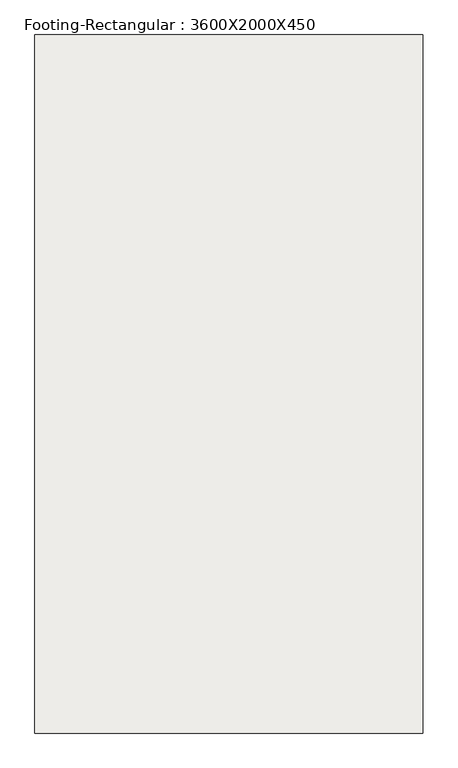
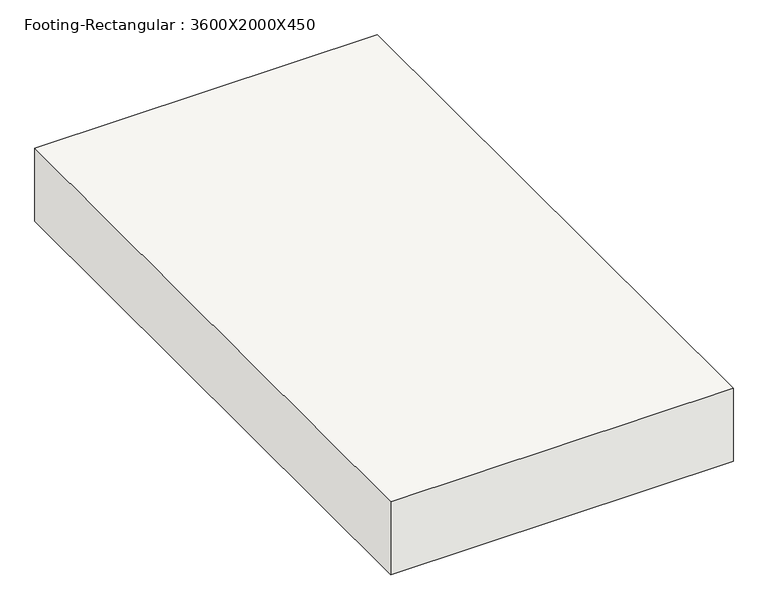
"""IFC4 building model written with IfcOpenShell, lengths in millimetres: slab geometry, Footing-Rectangular : 3600X2000X450."""

from ifc_helpers import new_model, si_unit, frame, origin, place, context, project, spatial, polyline, outline, extrude, source, transform, mapped, element, save


def footing_rectangular_3600x2000x450_36af6fae(model_context):
    return source(origin(), model_context, "Body", "SweptSolid", [
        extrude(outline(polyline([(1000.0, 1800.0), (1000.0, -1800.0), (-1000.0, -1800.0), (-1000.0, 1800.0), (1000.0, 1800.0)])), frame((0.0, 0.0, -450.0), z_axis=(0.0, 0.0, 1.0), x_axis=(1.0, 0.0, 0.0)), (0.0, 0.0, 1.0), 450.0),
    ])


if __name__ == "__main__":
    model = new_model("IFC4")
    model_context = context("Model", 3, world=origin())
    ifc_project = project(units=[si_unit("LENGTHUNIT", "METRE", prefix="MILLI")], contexts=[model_context])
    site = spatial("IfcSite", under=ifc_project)
    building = spatial("IfcBuilding", under=site)
    placement = place(None, origin())
    footing_rectangular_3600x2000x450_shape = footing_rectangular_3600x2000x450_36af6fae(model_context)
    element("IfcSlab", 1, ObjectType="Footing-Rectangular : 3600X2000X450", at=placement, inside=building, context=model_context, shape_type="MappedRepresentation", body=[
        mapped(footing_rectangular_3600x2000x450_shape, transform((0.0, 0.0, 0.0), x_axis=(1.0, 0.0, 0.0), y_axis=(0.0, 1.0, 0.0), z_axis=(0.0, 0.0, 1.0))),
    ])
    save(model, "model.ifc")

# Revit data of these elements
# Type "Footing-Rectangular : 3600X2000X450"
#   Width = 6' - 6.74016"
#   Length = 11' - 9.73228"
#   Foundation Thickness = 1' - 5.71654"
#   Structural Material [instance default] = Concrete - Cast-in-Place Concrete
#   Assembly Code = ""
# Element 1 (IfcSlab, "Footing-Rectangular : 3600X2000X450")
#   Materials on its faces: "Concrete - Cast-in-Place Concrete"
# Materials
#   "Concrete - Cast-in-Place Concrete": class "Concrete", colour RGB 192 192 192, transparency 0, Cost = 0
